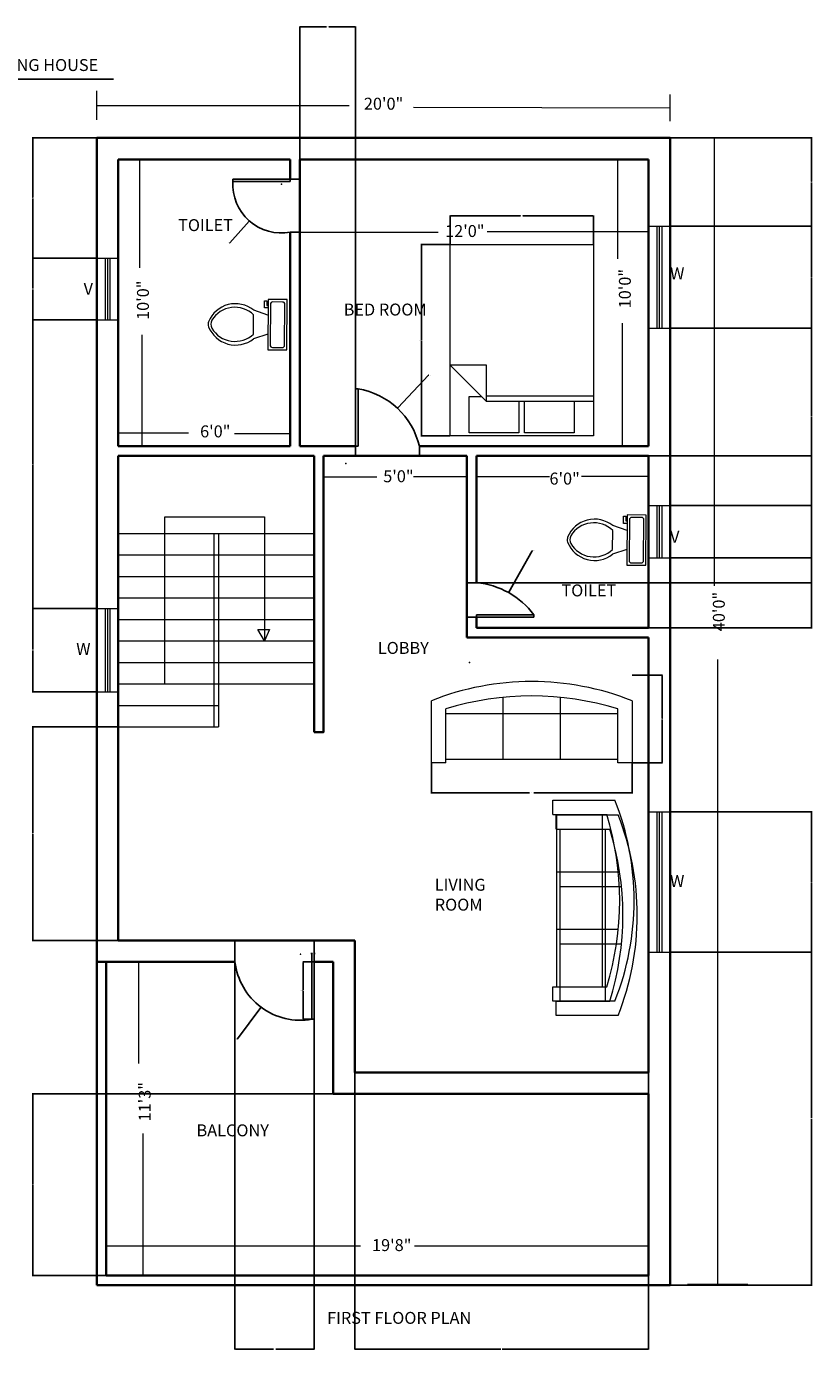
# Model space of a CAD drawing. Units: inches. Extents: x 37 to 686, y -425 to 128.
# Tile 3 of 3: x 357 to 686, y -425 to 128. Entities that reach past the tile are written whole.
import ezdxf

# ---------------------------------------------------------------- set-up
doc = ezdxf.new("R2010")
doc.units = ezdxf.units.IN
doc.header["$MEASUREMENT"] = 0
for name, color, linetype, lineweight in [('A-ANNO-DIMS', 2, 'Continuous', 13), ('A-ANNO-SYMB', 7, 'Continuous', 13), ('A-ANNO-TEXT', 7, 'Continuous', 18), ('A-ANNO-TITL', 7, 'Continuous', 25), ('A-AREA-IDEN', 7, 'Continuous', 18), ('A-DOOR', 3, 'Continuous', 25), ('A-FLOR-FIXT', 9, 'Continuous', 18), ('A-FLOR-STRS', 7, 'Continuous', 20), ('A-FURN', 8, 'Continuous', 18), ('A-GLAZ', 4, 'Continuous', 18), ('A-WALL', 7, 'Continuous', 35)]:
    doc.layers.add(name, color=color, linetype=linetype, lineweight=lineweight)
doc.styles.get("Standard").update_dxf_attribs({"font": 'arial.ttf'})
doc.dimstyles.get("Standard").update_dxf_attribs({"dimtxt": 0.18, "dimasz": 0.18, "dimexe": 0.18, "dimexo": 0.0625, "dimgap": 0.09, "dimtad": 0, "dimtih": 1, "dimtoh": 1, "dimdec": 4, "dimzin": 0, "dimdsep": 46, "dimtxsty": 'Standard', "dimcen": 0.09, "dimadec": 0, "dimazin": 0, "dimtfac": 1, "dimtdec": 4, "dimtofl": 0, "dimtmove": 0, "dimatfit": 3, "dimfxl": 1, "dimtolj": 1, "dimtzin": 0, "dimarcsym": 0})

# ---------------------------------------------------------------- blocks, each defined once
blk = doc.blocks.new('Bed - Queen')
for p, q in [((0, -80.00003), (0, 0)), ((0, 0), (59.99999, 0)), ((59.99999, 0), (59.99999, -80.00003)), ((7.99999, -1.2), (28.79998, -1.2)), ((7.99999, -14.4), (7.99999, -1.2)), ((28.79998, -1.2), (28.79998, -14.4)), ((31.19999, -1.2), (51.99999, -1.2)), ((31.19999, -14.4), (31.19999, -1.2)), ((51.99999, -1.2), (51.99999, -16.4)), ((0, -14.4), (44.8, -14.4)), ((59.99999, -29.6), (44.8, -14.4)), ((44.8, -14.4), (44.8, -29.6)), ((51.99999, -16.4), (46.79936, -16.4)), ((44.8, -16.8), (0, -16.8)), ((44.8, -29.6), (59.99999, -29.6)), ((59.99999, -80.00003), (0, -80.00003))]:
    blk.add_line(p, q)
blk = doc.blocks.new('Sofa - Roundback 7 ft.')
for p, q in [((-12.00002, -32.4421), (-12.00003, -6.5971)), ((11.99997, -32.4421), (11.99998, -6.5971)), ((-36.000027, -34), (-36.000027, -11.4696)), ((-35.999844, -13.3819), (35.9998, -13.3819)), ((35.99998, -34), (35.99998, -11.4696)), ((-36.000027, -32.4421), (35.99998, -32.4421))]:
    blk.add_line(p, q)
for points in [[(-36.000027, -34), (-42.000027, -34), (-42.000027, -8)], [(41.99998, -8), (41.99998, -34), (35.99998, -34)]]:
    blk.add_lwpolyline(points)
for centre, radius, start, end in [((0, -114.25), 114.25, 68.43141, 111.5686), ((-0.00001, -127.1968), 121.1968, 72.72033, 107.2797)]:
    blk.add_arc(centre, radius, start, end)
blk = doc.blocks.new('Toilet - top')
for p, q in [((9.5, -6), (9.5, -2)), ((-10, -8.5), (-8, -8.5)), ((-10, -9.5), (-10, -8.5)), ((-7, -9.5), (-10, -9.5)), ((-8, -8.5), (-8, -8)), ((-7, -8), (-7, -9.5)), ((-4, -8), (-6, -14)), ((4, -8), (6, -14)), ((4, -14), (-4, -14))]:
    blk.add_line(p, q)
blk.add_lwpolyline([(10.5, -8), (10.5, 0), (-10.5, 0), (-10.5, -8)], close=True)
for points in [[(-9.5, -2), (-9.5, -6)], [(8.5, -1), (-8.5, -1)], [(-8.5, -7), (8.5, -7)]]:
    blk.add_lwpolyline(points)
for centre, radius, start, end in [((-8.62, -1.88), 0.884, 81.8699, 188.1301), ((8.62, -1.88), 0.884, 351.8699, 98.1301), ((-8.62, -6.12), 0.884, 171.8699, 278.1301), ((8.62, -6.12), 0.884, 261.8699, 8.1301), ((3.52, -21.58), 12.17, 141.4691, 247.9714), ((4.2, -21.82), 11.33, 136.3677, 238.9468), ((-3.52, -21.58), 12.17, 292.0284, 38.5307), ((-4.2, -21.82), 11.33, 301.053, 43.6321), ((0, -27.88), 4, 245.7318, 294.2682), ((0, -29), 4, 254.8605, 285.1395)]:
    blk.add_arc(centre, radius, start, end)
blk = doc.blocks.new('DOOR-LEAF-24IN')
for p, q in [((0, 0), (0, 24)), ((0, 24), (1, 24)), ((1, 24), (1, 0)), ((1, 0), (0, 0))]:
    blk.add_line(p, q)
blk = doc.blocks.new('*D8')
at = {"layer": 'A-ANNO-DIMS', "color": 0, "lineweight": -2, "transparency": 16777216}
for p, q in [((534.26, 37.12), (522.14, 37.12)), ((522.32, 36.94), (522.32, -2.7)), ((522.32, -42.7), (522.32, -3.06)), ((534.26, -42.88), (522.14, -42.88))]:
    blk.add_line(p, q, dxfattribs=at)
at = {"layer": 'A-ANNO-DIMS', "color": 0, "transparency": 16777216}
for points in [[(522.29, 36.94), (522.35, 36.94), (522.32, 37.12)], [(522.29, -42.7), (522.35, -42.7), (522.32, -42.88)]]:
    blk.add_solid(points, dxfattribs=at)
at = {"layer": 'Defpoints', "color": 0, "transparency": 16777216}
for p in [(534.32, 37.12), (522.32, -42.88), (534.32, -42.88)]:
    blk.add_point(p, dxfattribs=at)
at = {"layer": 'A-ANNO-DIMS', "color": 0, "transparency": 16777216, "insert": (522.32, -2.88), "char_height": 0.18, "attachment_point": 5}
blk.add_mtext('\\A1;BED 80 TYP.', dxfattribs=at)
blk = doc.blocks.new('*D9')
at = {"layer": 'A-ANNO-DIMS', "color": 0, "lineweight": -2, "transparency": 16777216}
for p, q in [((534.32, 37.18), (534.32, 49.3)), ((534.5, 49.12), (563.79, 49.12)), ((594.14, 49.12), (564.85, 49.12)), ((594.32, 37.18), (594.32, 49.3))]:
    blk.add_line(p, q, dxfattribs=at)
at = {"layer": 'A-ANNO-DIMS', "color": 0, "transparency": 16777216}
for points in [[(534.5, 49.15), (534.5, 49.09), (534.32, 49.12)], [(594.14, 49.15), (594.14, 49.09), (594.32, 49.12)]]:
    blk.add_solid(points, dxfattribs=at)
at = {"layer": 'Defpoints', "color": 0, "transparency": 16777216}
for p in [(534.32, 49.12), (534.32, 37.12), (594.32, 37.12)]:
    blk.add_point(p, dxfattribs=at)
at = {"layer": 'A-ANNO-DIMS', "color": 0, "transparency": 16777216, "insert": (564.32, 49.12), "char_height": 0.18, "attachment_point": 5}
blk.add_mtext('\\A1;60 TYP.', dxfattribs=at)
blk = doc.blocks.new('*D12')
at = {"layer": 'A-ANNO-DIMS', "color": 0, "lineweight": -2, "transparency": 16777216}
for p, q in [((476.39, -263), (472.67, -263)), ((472.85, -263.18), (472.85, -274.81)), ((472.85, -286.82), (472.85, -275.18)), ((476.39, -287), (472.67, -287))]:
    blk.add_line(p, q, dxfattribs=at)
at = {"layer": 'A-ANNO-DIMS', "color": 0, "transparency": 16777216}
for points in [[(472.82, -263.18), (472.88, -263.18), (472.85, -263)], [(472.82, -286.82), (472.88, -286.82), (472.85, -287)]]:
    blk.add_solid(points, dxfattribs=at)
at = {"layer": 'Defpoints', "color": 0, "transparency": 16777216}
for p in [(476.45, -263), (472.85, -287), (476.45, -287)]:
    blk.add_point(p, dxfattribs=at)
at = {"layer": 'A-ANNO-DIMS', "color": 0, "transparency": 16777216, "insert": (472.85, -275), "char_height": 0.18, "attachment_point": 5}
blk.add_mtext('\\A1;DOOR LEAF 24 TYP.', dxfattribs=at)
blk = doc.blocks.new('*D13')
at = {"layer": 'A-ANNO-DIMS', "color": 0, "lineweight": -2, "transparency": 16777216}
for p, q in [((476.27, -259.4), (476.09, -259.4)), ((476.45, -262.93), (476.45, -259.22)), ((477.45, -262.93), (477.45, -259.22)), ((477.63, -259.4), (477.81, -259.4))]:
    blk.add_line(p, q, dxfattribs=at)
at = {"layer": 'A-ANNO-DIMS', "color": 0, "transparency": 16777216}
for points in [[(476.27, -259.37), (476.27, -259.43), (476.45, -259.4)], [(477.63, -259.37), (477.63, -259.43), (477.45, -259.4)]]:
    blk.add_solid(points, dxfattribs=at)
at = {"layer": 'Defpoints', "color": 0, "transparency": 16777216}
for p in [(476.45, -259.4), (476.45, -263), (477.45, -263)]:
    blk.add_point(p, dxfattribs=at)
at = {"layer": 'A-ANNO-DIMS', "color": 0, "transparency": 16777216, "insert": (476.95, -259.4), "char_height": 0.18, "attachment_point": 5}
blk.add_mtext('\\A1;1 TYP.', dxfattribs=at)
blk = doc.blocks.new('*D14')
at = {"layer": 'A-ANNO-DIMS', "color": 0, "lineweight": -2, "transparency": 16777216}
for p, q in [((526.49, -179.75), (526.49, -192.47)), ((610.49, -179.75), (610.49, -192.47)), ((526.67, -192.29), (567.59, -192.29)), ((610.31, -192.29), (569.4, -192.29))]:
    blk.add_line(p, q, dxfattribs=at)
at = {"layer": 'A-ANNO-DIMS', "color": 0, "transparency": 16777216}
for points in [[(526.67, -192.26), (526.67, -192.32), (526.49, -192.29)], [(610.31, -192.26), (610.31, -192.32), (610.49, -192.29)]]:
    blk.add_solid(points, dxfattribs=at)
at = {"layer": 'Defpoints', "color": 0, "transparency": 16777216}
for p in [(526.49, -179.69), (610.49, -179.69), (610.49, -192.29)]:
    blk.add_point(p, dxfattribs=at)
at = {"layer": 'A-ANNO-DIMS', "color": 0, "transparency": 16777216, "insert": (568.49, -192.29), "char_height": 0.18, "attachment_point": 5}
blk.add_mtext('\\A1;SOFA 84 TYP.', dxfattribs=at)
blk = doc.blocks.new('*D15')
at = {"layer": 'A-ANNO-DIMS', "color": 0, "lineweight": -2, "transparency": 16777216}
for p, q in [((610.55, -143.02), (623.27, -143.02)), ((623.09, -143.2), (623.09, -161.18)), ((623.09, -179.51), (623.09, -161.54)), ((610.55, -179.69), (623.27, -179.69))]:
    blk.add_line(p, q, dxfattribs=at)
at = {"layer": 'A-ANNO-DIMS', "color": 0, "transparency": 16777216}
for points in [[(623.06, -143.2), (623.12, -143.2), (623.09, -143.02)], [(623.06, -179.51), (623.12, -179.51), (623.09, -179.69)]]:
    blk.add_solid(points, dxfattribs=at)
at = {"layer": 'Defpoints', "color": 0, "transparency": 16777216}
for p in [(610.49, -143.02), (623.09, -143.02), (610.49, -179.69)]:
    blk.add_point(p, dxfattribs=at)
at = {"layer": 'A-ANNO-DIMS', "color": 0, "transparency": 16777216, "insert": (623.09, -161.36), "char_height": 0.18, "attachment_point": 5}
blk.add_mtext('\\A1;37 TYP.', dxfattribs=at)
blk = doc.blocks.new('*D26')
at = {"layer": 'A-ANNO-DIMS', "color": 0, "lineweight": -2, "transparency": 16777216}
for p, q in [((617.35, -318.23), (359.48, -318.23)), ((359.66, -318.41), (359.66, -356.05)), ((359.66, -394.05), (359.66, -356.41)), ((617.35, -394.23), (359.48, -394.23))]:
    blk.add_line(p, q, dxfattribs=at)
at = {"layer": 'A-ANNO-DIMS', "color": 0, "transparency": 16777216}
for points in [[(359.63, -318.41), (359.69, -318.41), (359.66, -318.23)], [(359.63, -394.05), (359.69, -394.05), (359.66, -394.23)]]:
    blk.add_solid(points, dxfattribs=at)
at = {"layer": 'Defpoints', "color": 0, "transparency": 16777216}
for p in [(617.41, -318.23), (359.66, -394.23), (617.41, -394.23)]:
    blk.add_point(p, dxfattribs=at)
at = {"layer": 'A-ANNO-DIMS', "color": 0, "transparency": 16777216, "insert": (359.66, -356.23), "char_height": 0.18, "attachment_point": 5}
blk.add_mtext('\\A1;76', dxfattribs=at)
blk = doc.blocks.new('*D27')
at = {"layer": 'A-ANNO-DIMS', "color": 0, "lineweight": -2, "transparency": 16777216}
for p, q in [((494.42, -309.29), (494.42, -425.16)), ((617.41, -309.29), (617.41, -425.16)), ((494.6, -424.98), (555.64, -424.98)), ((617.23, -424.98), (556.2, -424.98))]:
    blk.add_line(p, q, dxfattribs=at)
at = {"layer": 'A-ANNO-DIMS', "color": 0, "transparency": 16777216}
for points in [[(494.6, -424.95), (494.6, -425.01), (494.42, -424.98)], [(617.23, -424.95), (617.23, -425.01), (617.41, -424.98)]]:
    blk.add_solid(points, dxfattribs=at)
at = {"layer": 'Defpoints', "color": 0, "transparency": 16777216}
for p in [(494.42, -309.23), (617.41, -309.23), (617.41, -424.98)]:
    blk.add_point(p, dxfattribs=at)
at = {"layer": 'A-ANNO-DIMS', "color": 0, "transparency": 16777216, "insert": (555.92, -424.98), "char_height": 0.18, "attachment_point": 5}
blk.add_mtext('\\A1;123', dxfattribs=at)
blk = doc.blocks.new('*D28')
at = {"layer": 'A-ANNO-DIMS', "color": 0, "lineweight": -2, "transparency": 16777216}
for p, q in [((617.47, -51.23), (685.85, -51.23)), ((685.67, -51.41), (685.67, -87.05)), ((685.67, -123.05), (685.67, -87.41)), ((617.47, -123.23), (685.85, -123.23))]:
    blk.add_line(p, q, dxfattribs=at)
at = {"layer": 'A-ANNO-DIMS', "color": 0, "transparency": 16777216}
for points in [[(685.64, -51.41), (685.7, -51.41), (685.67, -51.23)], [(685.64, -123.05), (685.7, -123.05), (685.67, -123.23)]]:
    blk.add_solid(points, dxfattribs=at)
at = {"layer": 'Defpoints', "color": 0, "transparency": 16777216}
for p in [(617.41, -51.23), (617.41, -123.23), (685.67, -123.23)]:
    blk.add_point(p, dxfattribs=at)
at = {"layer": 'A-ANNO-DIMS', "color": 0, "transparency": 16777216, "insert": (685.67, -87.23), "char_height": 0.18, "attachment_point": 5}
blk.add_mtext('\\A1;72', dxfattribs=at)
blk = doc.blocks.new('*D36')
at = {"layer": 'A-ANNO-DIMS', "color": 0, "lineweight": -2, "transparency": 16777216}
for p, q in [((386.35, -115.05), (359.48, -115.05)), ((359.66, -115.23), (359.66, -132.33)), ((359.66, -149.79), (359.66, -132.69)), ((386.35, -149.97), (359.48, -149.97))]:
    blk.add_line(p, q, dxfattribs=at)
at = {"layer": 'A-ANNO-DIMS', "color": 0, "transparency": 16777216}
for points in [[(359.63, -115.23), (359.69, -115.23), (359.66, -115.05)], [(359.63, -149.79), (359.69, -149.79), (359.66, -149.97)]]:
    blk.add_solid(points, dxfattribs=at)
at = {"layer": 'Defpoints', "color": 0, "transparency": 16777216}
for p in [(359.66, -115.05), (386.41, -115.05), (386.41, -149.97)]:
    blk.add_point(p, dxfattribs=at)
at = {"layer": 'A-ANNO-DIMS', "color": 0, "transparency": 16777216, "insert": (359.66, -132.51), "char_height": 0.18, "attachment_point": 5}
blk.add_mtext('\\A1;34.91', dxfattribs=at)
blk = doc.blocks.new('*D37')
at = {"layer": 'A-ANNO-DIMS', "color": 0, "lineweight": -2, "transparency": 16777216}
for p, q in [((386.35, 31.44), (359.48, 31.44)), ((359.66, 31.26), (359.66, 18.71)), ((359.66, 5.8), (359.66, 18.35)), ((386.35, 5.62), (359.48, 5.62))]:
    blk.add_line(p, q, dxfattribs=at)
at = {"layer": 'A-ANNO-DIMS', "color": 0, "transparency": 16777216}
for points in [[(359.63, 31.26), (359.69, 31.26), (359.66, 31.44)], [(359.63, 5.8), (359.69, 5.8), (359.66, 5.62)]]:
    blk.add_solid(points, dxfattribs=at)
at = {"layer": 'Defpoints', "color": 0, "transparency": 16777216}
for p in [(359.66, 31.44), (386.41, 31.44), (386.41, 5.62)]:
    blk.add_point(p, dxfattribs=at)
at = {"layer": 'A-ANNO-DIMS', "color": 0, "transparency": 16777216, "insert": (359.66, 18.53), "char_height": 0.18, "attachment_point": 5}
blk.add_mtext('\\A1;25.823', dxfattribs=at)
blk = doc.blocks.new('*D38')
at = {"layer": 'A-ANNO-DIMS', "color": 0, "lineweight": -2, "transparency": 16777216}
for p, q in [((626.47, 44.9), (685.85, 44.9)), ((685.67, 44.72), (685.67, 23.7)), ((685.67, 2.31), (685.67, 23.34)), ((626.47, 2.13), (685.85, 2.13))]:
    blk.add_line(p, q, dxfattribs=at)
at = {"layer": 'A-ANNO-DIMS', "color": 0, "transparency": 16777216}
for points in [[(685.64, 44.72), (685.7, 44.72), (685.67, 44.9)], [(685.64, 2.31), (685.7, 2.31), (685.67, 2.13)]]:
    blk.add_solid(points, dxfattribs=at)
at = {"layer": 'Defpoints', "color": 0, "transparency": 16777216}
for p in [(626.41, 44.9), (685.67, 44.9), (626.41, 2.13)]:
    blk.add_point(p, dxfattribs=at)
at = {"layer": 'A-ANNO-DIMS', "color": 0, "transparency": 16777216, "insert": (685.67, 23.52), "char_height": 0.18, "attachment_point": 5}
blk.add_mtext('\\A1;42.77', dxfattribs=at)
blk = doc.blocks.new('*D39')
at = {"layer": 'A-ANNO-DIMS', "color": 0, "lineweight": -2, "transparency": 16777216}
for p, q in [((626.47, -71.98), (685.85, -71.98)), ((685.67, -72.16), (685.67, -82.77)), ((685.67, -93.75), (685.67, -83.14)), ((626.47, -93.93), (685.85, -93.93))]:
    blk.add_line(p, q, dxfattribs=at)
at = {"layer": 'A-ANNO-DIMS', "color": 0, "transparency": 16777216}
for points in [[(685.64, -72.16), (685.7, -72.16), (685.67, -71.98)], [(685.64, -93.75), (685.7, -93.75), (685.67, -93.93)]]:
    blk.add_solid(points, dxfattribs=at)
at = {"layer": 'Defpoints', "color": 0, "transparency": 16777216}
for p in [(626.41, -71.98), (626.41, -93.93), (685.67, -93.93)]:
    blk.add_point(p, dxfattribs=at)
at = {"layer": 'A-ANNO-DIMS', "color": 0, "transparency": 16777216, "insert": (685.67, -82.95), "char_height": 0.18, "attachment_point": 5}
blk.add_mtext('\\A1;21.946', dxfattribs=at)
blk = doc.blocks.new('*D40')
at = {"layer": 'A-ANNO-DIMS', "color": 0, "lineweight": -2, "transparency": 16777216}
for p, q in [((626.47, -200.25), (685.85, -200.25)), ((685.67, -200.43), (685.67, -229.42)), ((685.67, -258.77), (685.67, -229.79)), ((626.47, -258.95), (685.85, -258.95))]:
    blk.add_line(p, q, dxfattribs=at)
at = {"layer": 'A-ANNO-DIMS', "color": 0, "transparency": 16777216}
for points in [[(685.64, -200.43), (685.7, -200.43), (685.67, -200.25)], [(685.64, -258.77), (685.7, -258.77), (685.67, -258.95)]]:
    blk.add_solid(points, dxfattribs=at)
at = {"layer": 'Defpoints', "color": 0, "transparency": 16777216}
for p in [(626.41, -200.25), (685.67, -200.25), (626.41, -258.95)]:
    blk.add_point(p, dxfattribs=at)
at = {"layer": 'A-ANNO-DIMS', "color": 0, "transparency": 16777216, "insert": (685.67, -229.6), "char_height": 0.18, "attachment_point": 5}
blk.add_mtext('\\A1;58.7', dxfattribs=at)
blk = doc.blocks.new('*D48')
at = {"layer": 'A-ANNO-DIMS', "color": 0, "lineweight": -2, "transparency": 16777216}
for p, q in [((386.35, 81.77), (359.48, 81.77)), ((359.66, 81.59), (359.66, 56.79)), ((359.66, 31.62), (359.66, 56.42)), ((386.35, 31.44), (359.48, 31.44))]:
    blk.add_line(p, q, dxfattribs=at)
at = {"layer": 'A-ANNO-DIMS', "color": 0, "transparency": 16777216}
for points in [[(359.63, 81.59), (359.69, 81.59), (359.66, 81.77)], [(359.63, 31.62), (359.69, 31.62), (359.66, 31.44)]]:
    blk.add_solid(points, dxfattribs=at)
at = {"layer": 'Defpoints', "color": 0, "transparency": 16777216}
for p in [(359.66, 81.77), (386.41, 81.77), (386.41, 31.44)]:
    blk.add_point(p, dxfattribs=at)
at = {"layer": 'A-ANNO-DIMS', "color": 0, "transparency": 16777216, "insert": (359.66, 56.61), "char_height": 0.18, "attachment_point": 5}
blk.add_mtext('\\A1;50.33', dxfattribs=at)
blk = doc.blocks.new('*D49')
at = {"layer": 'A-ANNO-DIMS', "color": 0, "lineweight": -2, "transparency": 16777216}
for p, q in [((386.35, 5.62), (359.48, 5.62)), ((359.66, 5.44), (359.66, -54.54)), ((359.66, -114.87), (359.66, -54.9)), ((386.35, -115.05), (359.48, -115.05))]:
    blk.add_line(p, q, dxfattribs=at)
at = {"layer": 'A-ANNO-DIMS', "color": 0, "transparency": 16777216}
for points in [[(359.63, 5.44), (359.69, 5.44), (359.66, 5.62)], [(359.63, -114.87), (359.69, -114.87), (359.66, -115.05)]]:
    blk.add_solid(points, dxfattribs=at)
at = {"layer": 'Defpoints', "color": 0, "transparency": 16777216}
for p in [(359.66, 5.62), (386.41, 5.62), (386.41, -115.05)]:
    blk.add_point(p, dxfattribs=at)
at = {"layer": 'A-ANNO-DIMS', "color": 0, "transparency": 16777216, "insert": (359.66, -54.72), "char_height": 0.18, "attachment_point": 5}
blk.add_mtext('\\A1;120.67', dxfattribs=at)
blk = doc.blocks.new('*D50')
at = {"layer": 'A-ANNO-DIMS', "color": 0, "lineweight": -2, "transparency": 16777216}
for p, q in [((626.47, 81.77), (685.85, 81.77)), ((685.67, 81.59), (685.67, 63.52)), ((685.67, 45.08), (685.67, 63.16)), ((626.47, 44.9), (685.85, 44.9))]:
    blk.add_line(p, q, dxfattribs=at)
at = {"layer": 'A-ANNO-DIMS', "color": 0, "transparency": 16777216}
for points in [[(685.64, 81.59), (685.7, 81.59), (685.67, 81.77)], [(685.64, 45.08), (685.7, 45.08), (685.67, 44.9)]]:
    blk.add_solid(points, dxfattribs=at)
at = {"layer": 'Defpoints', "color": 0, "transparency": 16777216}
for p in [(626.41, 81.77), (685.67, 81.77), (626.41, 44.9)]:
    blk.add_point(p, dxfattribs=at)
at = {"layer": 'A-ANNO-DIMS', "color": 0, "transparency": 16777216, "insert": (685.67, 63.34), "char_height": 0.18, "attachment_point": 5}
blk.add_mtext('\\A1;36.87', dxfattribs=at)
blk = doc.blocks.new('*D51')
at = {"layer": 'A-ANNO-DIMS', "color": 0, "lineweight": -2, "transparency": 16777216}
for p, q in [((626.47, 2.13), (685.85, 2.13)), ((685.67, 1.95), (685.67, -34.74)), ((685.67, -71.8), (685.67, -35.1)), ((626.47, -71.98), (685.85, -71.98))]:
    blk.add_line(p, q, dxfattribs=at)
at = {"layer": 'A-ANNO-DIMS', "color": 0, "transparency": 16777216}
for points in [[(685.64, 1.95), (685.7, 1.95), (685.67, 2.13)], [(685.64, -71.8), (685.7, -71.8), (685.67, -71.98)]]:
    blk.add_solid(points, dxfattribs=at)
at = {"layer": 'Defpoints', "color": 0, "transparency": 16777216}
for p in [(626.41, 2.13), (685.67, 2.13), (626.41, -71.98)]:
    blk.add_point(p, dxfattribs=at)
at = {"layer": 'A-ANNO-DIMS', "color": 0, "transparency": 16777216, "insert": (685.67, -34.92), "char_height": 0.18, "attachment_point": 5}
blk.add_mtext('\\A1;74.11', dxfattribs=at)
blk = doc.blocks.new('*D52')
at = {"layer": 'A-ANNO-DIMS', "color": 0, "lineweight": -2, "transparency": 16777216}
for p, q in [((626.47, -258.95), (685.85, -258.95)), ((685.67, -259.13), (685.67, -328.41)), ((685.67, -398.05), (685.67, -328.77)), ((626.47, -398.23), (685.85, -398.23))]:
    blk.add_line(p, q, dxfattribs=at)
at = {"layer": 'A-ANNO-DIMS', "color": 0, "transparency": 16777216}
for points in [[(685.64, -259.13), (685.7, -259.13), (685.67, -258.95)], [(685.64, -398.05), (685.7, -398.05), (685.67, -398.23)]]:
    blk.add_solid(points, dxfattribs=at)
at = {"layer": 'Defpoints', "color": 0, "transparency": 16777216}
for p in [(626.41, -258.95), (685.67, -258.95), (626.41, -398.23)]:
    blk.add_point(p, dxfattribs=at)
at = {"layer": 'A-ANNO-DIMS', "color": 0, "transparency": 16777216, "insert": (685.67, -328.59), "char_height": 0.18, "attachment_point": 5}
blk.add_mtext('\\A1;139.27', dxfattribs=at)
blk = doc.blocks.new('*D55')
at = {"layer": 'A-ANNO-DIMS', "color": 0, "lineweight": -2, "transparency": 16777216}
for p, q in [((444.29, -263.06), (444.29, -425.16)), ((477.45, -263.06), (477.45, -425.16)), ((444.47, -424.98), (460.41, -424.98)), ((477.27, -424.98), (461.34, -424.98))]:
    blk.add_line(p, q, dxfattribs=at)
at = {"layer": 'A-ANNO-DIMS', "color": 0, "transparency": 16777216}
for points in [[(444.47, -424.95), (444.47, -425.01), (444.29, -424.98)], [(477.27, -424.95), (477.27, -425.01), (477.45, -424.98)]]:
    blk.add_solid(points, dxfattribs=at)
at = {"layer": 'Defpoints', "color": 0, "transparency": 16777216}
for p in [(444.29, -263), (477.45, -263), (477.45, -424.98)]:
    blk.add_point(p, dxfattribs=at)
at = {"layer": 'A-ANNO-DIMS', "color": 0, "transparency": 16777216, "insert": (460.87, -424.98), "char_height": 0.18, "attachment_point": 5}
blk.add_mtext('\\A1;33.156', dxfattribs=at)
blk = doc.blocks.new('*D56')
at = {"layer": 'A-ANNO-DIMS', "color": 0, "lineweight": -2, "transparency": 16777216}
for p, q in [((395.35, -164.68), (359.48, -164.68)), ((359.66, -164.86), (359.66, -209.15)), ((359.66, -253.82), (359.66, -209.52)), ((395.35, -254), (359.48, -254))]:
    blk.add_line(p, q, dxfattribs=at)
at = {"layer": 'A-ANNO-DIMS', "color": 0, "transparency": 16777216}
for points in [[(359.63, -164.86), (359.69, -164.86), (359.66, -164.68)], [(359.63, -253.82), (359.69, -253.82), (359.66, -254)]]:
    blk.add_solid(points, dxfattribs=at)
at = {"layer": 'Defpoints', "color": 0, "transparency": 16777216}
for p in [(359.66, -164.68), (395.41, -164.68), (395.41, -254)]:
    blk.add_point(p, dxfattribs=at)
at = {"layer": 'A-ANNO-DIMS', "color": 0, "transparency": 16777216, "insert": (359.66, -209.34), "char_height": 0.18, "attachment_point": 5}
blk.add_mtext('\\A1;89.32', dxfattribs=at)
blk = doc.blocks.new('*D60')
at = {"layer": 'A-ANNO-DIMS', "color": 0, "lineweight": -2, "transparency": 16777216}
for p, q in [((471.41, -47.16), (471.41, 128.4)), ((471.59, 128.22), (482.64, 128.22)), ((494.62, 128.22), (483.57, 128.22)), ((494.8, -47.16), (494.8, 128.4))]:
    blk.add_line(p, q, dxfattribs=at)
at = {"layer": 'A-ANNO-DIMS', "color": 0, "transparency": 16777216}
for points in [[(471.59, 128.25), (471.59, 128.19), (471.41, 128.22)], [(494.62, 128.25), (494.62, 128.19), (494.8, 128.22)]]:
    blk.add_solid(points, dxfattribs=at)
at = {"layer": 'Defpoints', "color": 0, "transparency": 16777216}
for p in [(494.8, 128.22), (471.41, -47.23), (494.8, -47.23)]:
    blk.add_point(p, dxfattribs=at)
at = {"layer": 'A-ANNO-DIMS', "color": 0, "transparency": 16777216, "insert": (483.1, 128.22), "char_height": 0.18, "attachment_point": 5}
blk.add_mtext('\\A1;23.386', dxfattribs=at)
blk = doc.blocks.new('*D61')
at = {"layer": 'A-ANNO-DIMS', "color": 0, "lineweight": -2, "transparency": 16777216}
for p, q in [((545.47, -51.23), (685.85, -51.23)), ((685.67, -51.41), (685.67, -77.59)), ((685.67, -104.14), (685.67, -77.95)), ((545.47, -104.32), (685.85, -104.32))]:
    blk.add_line(p, q, dxfattribs=at)
at = {"layer": 'A-ANNO-DIMS', "color": 0, "transparency": 16777216}
for points in [[(685.64, -51.41), (685.7, -51.41), (685.67, -51.23)], [(685.64, -104.14), (685.7, -104.14), (685.67, -104.32)]]:
    blk.add_solid(points, dxfattribs=at)
at = {"layer": 'Defpoints', "color": 0, "transparency": 16777216}
for p in [(545.41, -51.23), (545.41, -104.32), (685.67, -104.32)]:
    blk.add_point(p, dxfattribs=at)
at = {"layer": 'A-ANNO-DIMS', "color": 0, "transparency": 16777216, "insert": (685.67, -77.77), "char_height": 0.18, "attachment_point": 5}
blk.add_mtext('\\A1;53.09', dxfattribs=at)
blk = doc.blocks.new('*D63')
at = {"layer": 'A-ANNO-DIMS', "color": 0, "lineweight": -2, "transparency": 16777216}
for p, q in [((568.71, -90.95), (558.95, -108.33)), ((568.89, -90.95), (568.71, -90.95)), ((542.35, -137.71), (542.53, -137.71)), ((542.44, -137.8), (542.44, -137.62))]:
    blk.add_line(p, q, dxfattribs=at)
at = {"layer": 'A-ANNO-DIMS', "color": 0, "transparency": 16777216}
blk.add_solid([(558.92, -108.31), (558.97, -108.34), (558.86, -108.48)], dxfattribs=at)
at = {"layer": 'Defpoints', "color": 0, "transparency": 16777216}
for p in [(558.86, -108.48), (542.44, -137.71)]:
    blk.add_point(p, dxfattribs=at)
at = {"layer": 'A-ANNO-DIMS', "color": 0, "transparency": 16777216, "insert": (569.37, -90.95), "char_height": 0.18, "attachment_point": 5}
blk.add_mtext('\\A1;R33.52', dxfattribs=at)
blk = doc.blocks.new('*D65')
at = {"layer": 'A-ANNO-DIMS', "color": 0, "lineweight": -2, "transparency": 16777216}
for p, q in [((525.24, -17.46), (512.41, -31.2)), ((525.42, -17.46), (525.24, -17.46)), ((490.61, -54.44), (490.79, -54.44)), ((490.7, -54.53), (490.7, -54.35))]:
    blk.add_line(p, q, dxfattribs=at)
at = {"layer": 'A-ANNO-DIMS', "color": 0, "transparency": 16777216}
blk.add_solid([(512.39, -31.18), (512.43, -31.22), (512.29, -31.33)], dxfattribs=at)
at = {"layer": 'Defpoints', "color": 0, "transparency": 16777216}
for p in [(512.29, -31.33), (490.7, -54.44)]:
    blk.add_point(p, dxfattribs=at)
at = {"layer": 'A-ANNO-DIMS', "color": 0, "transparency": 16777216, "insert": (525.9, -17.46), "char_height": 0.18, "attachment_point": 5}
blk.add_mtext('\\A1;R31.62', dxfattribs=at)
blk = doc.blocks.new('*D67')
at = {"layer": 'A-ANNO-DIMS', "color": 0, "lineweight": -2, "transparency": 16777216}
for p, q in [((471.65, -259.77), (471.83, -259.77)), ((471.74, -259.86), (471.74, -259.68)), ((445.29, -295.2), (455.1, -282.06)), ((445.11, -295.2), (445.29, -295.2))]:
    blk.add_line(p, q, dxfattribs=at)
at = {"layer": 'A-ANNO-DIMS', "color": 0, "transparency": 16777216}
blk.add_solid([(455.08, -282.04), (455.13, -282.07), (455.21, -281.91)], dxfattribs=at)
at = {"layer": 'Defpoints', "color": 0, "transparency": 16777216}
for p in [(471.74, -259.77), (455.21, -281.91)]:
    blk.add_point(p, dxfattribs=at)
at = {"layer": 'A-ANNO-DIMS', "color": 0, "transparency": 16777216, "insert": (444.63, -295.2), "char_height": 0.18, "attachment_point": 5}
blk.add_mtext('\\A1;R27.63', dxfattribs=at)
blk = doc.blocks.new('*D69')
at = {"layer": 'A-ANNO-DIMS', "color": 0, "lineweight": -2, "transparency": 16777216}
for p, q in [((463.69, 62.4), (463.87, 62.4)), ((463.78, 62.31), (463.78, 62.49)), ((442.19, 37.92), (450.17, 46.96)), ((442.01, 37.92), (442.19, 37.92))]:
    blk.add_line(p, q, dxfattribs=at)
at = {"layer": 'A-ANNO-DIMS', "color": 0, "transparency": 16777216}
blk.add_solid([(450.14, 46.98), (450.19, 46.94), (450.29, 47.1)], dxfattribs=at)
at = {"layer": 'Defpoints', "color": 0, "transparency": 16777216}
for p in [(463.78, 62.4), (450.29, 47.1)]:
    blk.add_point(p, dxfattribs=at)
at = {"layer": 'A-ANNO-DIMS', "color": 0, "transparency": 16777216, "insert": (441.46, 37.92), "char_height": 0.18, "attachment_point": 5}
blk.add_mtext('\\A1;R20.402', dxfattribs=at)

msp = doc.modelspace()

# ---------------------------------------------------------------- linework, layer by layer
at = {"layer": 'A-ANNO-DIMS'}
for p, q in [((386.4114, 89.3296), (386.4114, 101.4672)), ((626.4114, 88.7375), (626.4114, 99.987)), ((386.4114, 95.3984), (492.0307, 95.3984)), ((519.0018, 94.6583), (626.4114, 94.3623)), ((631.909, 81.9543), (657.8745, 81.9543)), ((644.8918, 81.9543), (644.8918, -105.6438)), ((404.4762, 27.441), (404.4762, 72.7729)), ((604.4594, 72.7729), (604.4594, 31.1608)), ((471.4114, 42.3205), (529.3772, 42.3205)), ((549.8488, 42.6387), (617.4114, 42.6387)), ((606.29, 4.1919), (606.29, -47.2271)), ((405.3539, -0.6131), (405.3539, -47.2271)), ((424.7969, -41.7157), (395.4114, -41.7157)), ((444.0844, -41.841), (467.4114, -41.841)), ((481.4114, -60.0408), (503.6246, -60.0408)), ((519.0833, -59.8976), (541.4114, -59.8976)), ((545.4114, -59.8976), (575.9323, -59.8976)), ((589.3506, -59.6849), (617.4114, -59.6849)), ((646.3442, -397.7918), (646.3442, -136.4803)), ((404.018, -305.5393), (404.018, -262.9952)), ((405.7754, -334.764), (405.7754, -381.9605)), ((519.3979, -381.7828), (617.4114, -381.7828)), ((395.4114, -381.9605), (390.4114, -381.9605)), ((496.8886, -381.9605), (395.4114, -381.9605)), ((405.7754, -381.9605), (405.7754, -389.2271)), ((405.7754, -389.2271), (405.7754, -394.2271)), ((633.7697, -397.7918), (658.9186, -397.7918))]:
    msp.add_line(p, q, dxfattribs=at)
at = {"layer": 'A-ANNO-SYMB'}
for p, q in [((414.9345, -146.6754), (414.9345, -76.746)), ((414.9345, -76.746), (456.6656, -76.746)), ((456.6656, -76.746), (456.6656, -128.6754)), ((456.6656, -128.6754), (453.9181, -123.9166)), ((453.9181, -123.9166), (458.8028, -123.9166)), ((458.8028, -123.9166), (456.6656, -128.6754))]:
    msp.add_line(p, q, dxfattribs=at)
at = {"layer": 'A-ANNO-TITL'}
msp.add_line((320.568, 106.3633), (393.4497, 106.3633), dxfattribs=at)
at = {"layer": 'A-DOOR'}
for p, q in [((467.4114, 64.4949), (471.4114, 64.4949)), ((467.4114, 42.3205), (471.4114, 42.3205)), ((494.7972, -51.2271), (494.7972, -47.2271)), ((521.4891, -51.2271), (521.4891, -47.2271)), ((541.4114, -104.3183), (545.4114, -104.3183)), ((541.4114, -118.8056), (545.4114, -118.8056)), ((444.2945, -262.9952), (444.2945, -253.9952)), ((477.4503, -262.9952), (477.4503, -253.9952))]:
    msp.add_line(p, q, dxfattribs=at)
for centre, radius, start, end in [((463.7844, 62.398), 20.4025, 176.918049, 280.240214), ((490.6991, -54.4361), 31.6227, 13.17759, 80.722384), ((542.4368, -137.7087), 33.5226, 36.421615, 84.909158), ((471.7376, -259.7679), 27.6322, 186.707299, 279.819796)]:
    msp.add_arc(centre, radius, start, end, dxfattribs=at)
at = {"layer": 'A-FLOR-STRS'}
for p, q in [((395.4114, -83.6754), (477.4114, -83.6754)), ((435.4114, -83.6754), (435.4114, -164.6754)), ((437.4114, -83.6754), (437.4114, -164.6754)), ((395.4114, -92.6754), (477.4114, -92.6754)), ((395.4114, -101.6754), (477.4114, -101.6754)), ((395.4114, -110.6754), (477.4114, -110.6754)), ((395.4114, -119.6754), (477.4114, -119.6754)), ((395.4114, -128.6754), (477.4114, -128.6754)), ((395.4114, -137.6754), (477.4114, -137.6754)), ((395.4114, -146.6754), (477.4114, -146.6754)), ((395.4114, -155.6754), (437.4114, -155.6754)), ((395.4114, -164.6754), (437.4114, -164.6754))]:
    msp.add_line(p, q, dxfattribs=at)
at = {"layer": 'A-GLAZ'}
for p, q in [((617.4114, 44.9049), (626.4114, 44.9049)), ((620.9114, 44.9049), (620.9114, 2.1316)), ((621.9114, 44.9049), (621.9114, 2.1316)), ((622.9114, 44.9049), (622.9114, 2.1316)), ((386.4114, 31.44), (395.4114, 31.44)), ((389.9114, 31.44), (389.9114, 5.6174)), ((390.9114, 31.44), (390.9114, 5.6174)), ((391.9114, 31.44), (391.9114, 5.6174)), ((386.4114, 5.6174), (395.4114, 5.6174)), ((617.4114, 2.1316), (626.4114, 2.1316)), ((617.4114, -71.9808), (626.4114, -71.9808)), ((620.9114, -71.9808), (620.9114, -93.9265)), ((621.9114, -71.9808), (621.9114, -93.9265)), ((622.9114, -71.9808), (622.9114, -93.9265)), ((617.4114, -93.9265), (626.4114, -93.9265)), ((386.4114, -115.0549), (395.4114, -115.0549)), ((389.9114, -115.0549), (389.9114, -149.9657)), ((390.9114, -115.0549), (390.9114, -149.9657)), ((391.9114, -115.0549), (391.9114, -149.9657)), ((386.4114, -149.9657), (395.4114, -149.9657)), ((617.4114, -200.252), (626.4114, -200.252)), ((620.9114, -200.252), (620.9114, -258.9544)), ((621.9114, -200.252), (621.9114, -258.9544)), ((622.9114, -200.252), (622.9114, -258.9544)), ((617.4114, -258.9544), (626.4114, -258.9544))]:
    msp.add_line(p, q, dxfattribs=at)
at = {"layer": 'A-WALL'}
for p, q in [((386.4114, 81.7729), (626.4114, 81.7729)), ((386.4114, -398.2271), (386.4114, 81.7729)), ((626.4114, 81.7729), (626.4114, -398.2271)), ((395.4114, 72.7729), (467.4114, 72.7729)), ((395.4114, -47.2271), (395.4114, 72.7729)), ((467.4114, 64.4949), (467.4114, 72.7729)), ((471.4114, -47.2271), (471.4114, 72.7729)), ((471.4114, 72.7729), (617.4114, 72.7729)), ((617.4114, 72.7729), (617.4114, -47.2271)), ((467.4114, -47.2271), (467.4114, 42.3205)), ((395.4114, -47.2271), (467.4114, -47.2271)), ((471.4114, -47.2271), (494.7972, -47.2271)), ((521.4891, -47.2271), (617.4114, -47.2271)), ((395.4114, -51.2271), (477.4114, -51.2271)), ((395.4114, -253.9952), (395.4114, -51.2271)), ((477.4114, -51.2271), (477.4114, -127.2271)), ((481.4114, -51.2271), (481.4114, -127.2271)), ((481.4114, -51.2271), (541.4114, -51.2271)), ((541.4114, -51.2271), (541.4114, -127.2271)), ((545.4114, -51.2271), (545.4114, -104.3183)), ((545.4114, -51.2271), (617.4114, -51.2271)), ((617.4114, -51.2271), (617.4114, -123.2271)), ((545.4114, -118.8056), (545.4114, -123.2271)), ((477.4114, -127.2271), (477.4114, -166.8153)), ((541.4114, -127.2271), (617.4114, -127.2271)), ((545.4114, -123.2271), (617.4114, -123.2271)), ((617.4114, -127.2271), (617.4114, -309.2271)), ((395.4114, -253.9952), (494.423, -253.9952)), ((494.423, -253.9952), (494.423, -309.2271)), ((395.4114, -262.9952), (386.4114, -262.9952)), ((390.4114, -394.2271), (390.4114, -262.9952)), ((395.4114, -262.9952), (444.2945, -262.9952)), ((477.4503, -262.9952), (485.423, -262.9952)), ((485.423, -262.9952), (485.423, -309.2271)), ((485.423, -309.2271), (485.423, -318.2271)), ((617.4114, -309.2271), (494.423, -309.2271)), ((617.4114, -318.2271), (485.423, -318.2271)), ((617.4114, -318.2271), (617.4114, -389.2271)), ((617.4114, -389.2271), (617.4114, -394.2271)), ((626.4114, -398.2271), (386.4114, -398.2271)), ((617.4114, -394.2271), (390.4114, -394.2271))]:
    msp.add_line(p, q, dxfattribs=at)
msp.add_lwpolyline([(481.4114, -127.2271), (481.4114, -166.8153), (477.4114, -166.8153)], dxfattribs=at)

# ---------------------------------------------------------------- block references
at = {"layer": 'A-DOOR'}
for p, rotation in [((443.4116, 64.4948), 269.9999999999999), ((569.4113, -118.8054), 89.99999999999984), ((477.4501, -262.9953), 180)]:
    msp.add_blockref('DOOR-LEAF-24IN', p, dxfattribs=dict(at, rotation=rotation))
msp.add_blockref('DOOR-LEAF-24IN', (494.7974, -47.227), dxfattribs=at)
at = {"layer": 'A-FLOR-FIXT', "rotation": 269.5733184257299}
for p in [(466.0881, 3.5942), (616.3761, -86.558)]:
    msp.add_blockref('Toilet - top', p, dxfattribs=at)
at = {"layer": 'A-FURN'}
for name, p, rotation in [('Bed - Queen', (594.3209, -42.8782), 180), ('Sofa - Roundback 7 ft.', (611.3478, -237.3424), 270), ('Sofa - Roundback 7 ft.', (612.6781, -243.4369), 270)]:
    msp.add_blockref(name, p, dxfattribs=dict(at, rotation=rotation))
msp.add_blockref('Sofa - Roundback 7 ft.', (568.4909, -145.6904), dxfattribs=at)

# ---------------------------------------------------------------- texts
at = {"layer": 'A-ANNO-DIMS', "char_height": 5, "attachment_point": 1}
for s, width, insert in [('20\'0"', 66.49393, (498.2548, 98.5799)), ('12\'0"', 35.858568, (532.2586, 45.3112)), ('6\'0"', 27.670391, (429.7013, -38.5194)), ('5\'0"', 20.747672, (506.3583, -57.2907)), ('6\'0"', 27.670391, (575.9323, -58.2717)), ('19\'8"', 40.826541, (501.665, -378.967))]:
    msp.add_mtext_dynamic_manual_height_columns(s, width=width, gutter_width=25, heights=[0], dxfattribs=dict(at, insert=insert))
at = {"layer": 'A-ANNO-DIMS', "char_height": 5, "attachment_point": 1, "rotation": 90}
for s, width, insert in [('10\'0"', 27.842625, (604.9853, 10.4667)), ('10\'0"', 27.842625, (403.2861, 5.6174)), ('40\'0"', 31.535776, (644.3193, -124.6216)), ('11\'3"', 24.184865, (404.018, -329.7241))]:
    msp.add_mtext_dynamic_manual_height_columns(s, width=width, gutter_width=25, heights=[0], dxfattribs=dict(at, insert=insert))
at = {"layer": 'A-ANNO-TEXT', "char_height": 5, "attachment_point": 1}
for s, width, insert in [('W', 8.568355, (626.4114, 27.5575)), ('V', 13.447234, (380.9472, 21.1263)), ('V', 13.447234, (626.4114, -82.6031)), ('W', 8.568355, (377.8535, -129.525)), ('W', 8.568355, (626.4114, -226.6384))]:
    msp.add_mtext_dynamic_manual_height_columns(s, width=width, gutter_width=25, heights=[0], dxfattribs=dict(at, insert=insert))
at = {"layer": 'A-ANNO-TITL', "char_height": 5, "attachment_point": 1}
for s, width, insert in [('EAST FACING HOUSE', 258.611498, (320.7609, 114.7635)), ('FIRST FLOOR PLAN', 184.056372, (482.8707, -409.4107))]:
    msp.add_mtext_dynamic_manual_height_columns(s, width=width, gutter_width=25, heights=[0], dxfattribs=dict(at, insert=insert))
at = {"layer": 'A-AREA-IDEN', "char_height": 5, "attachment_point": 1}
for s, width, insert in [('TOILET', 38.596876, (420.5149, 47.7824)), ('BED ROOM', 83.955241, (489.805, 12.4565)), ('TOILET', 38.596876, (580.9403, -105.0553)), ('LOBBY', 26.091096, (504.0968, -129.1153)), ('LIVING\\PROOM', 48.553453, (527.925, -228.1916)), ('BALCONY', 94.333055, (428.2028, -330.9559))]:
    msp.add_mtext_dynamic_manual_height_columns(s, width=width, gutter_width=25, heights=[0], dxfattribs=dict(at, insert=insert))

# ---------------------------------------------------------------- dimensions: what is measured, and where the dimension line sits
at = {"layer": 'A-ANNO-DIMS'}
for base, p1, p2, override, picture, middle in [((494.7972, 128.2172), (471.4114, -47.2271), (494.7972, -47.2271), {"dimdec": 3, "dimlfac": 1, "dimrnd": 0, "dimzin": 0, "dimdsep": 46, "dimlunit": 2}, '*D60', (483.1043, 128.2172)), ((477.4503, -424.9771), (444.2945, -262.9952), (477.4503, -262.9952), {"dimdec": 3, "dimlfac": 1, "dimrnd": 0, "dimzin": 0, "dimdsep": 46, "dimlunit": 2}, '*D55', (460.8724, -424.9771)), ((617.4114, -424.9771), (494.423, -309.2271), (617.4114, -309.2271), {"dimdec": 0, "dimlfac": 1, "dimrnd": 0, "dimzin": 0, "dimdsep": 46, "dimlunit": 2}, '*D27', (555.9172, -424.9771))]:
    dim = msp.add_linear_dim(base=base, p1=p1, p2=p2, dimstyle='Standard', override=override, dxfattribs=at)
    dim.commit()
    dim.dimension.update_dxf_attribs({"geometry": picture, "text_midpoint": middle})
for base, p1, p2, override, picture, middle in [((359.6614, 81.7729), (386.4114, 31.44), (386.4114, 81.7729), {"dimdec": 2, "dimlfac": 1, "dimrnd": 0, "dimzin": 0, "dimdsep": 46, "dimlunit": 2}, '*D48', (359.6614, 56.6064)), ((685.6686, 81.7729), (626.4114, 44.9049), (626.4114, 81.7729), {"dimdec": 2, "dimlfac": 1, "dimrnd": 0, "dimzin": 0, "dimdsep": 46, "dimlunit": 2}, '*D50', (685.6686, 63.3389)), ((685.6686, 44.9049), (626.4114, 2.1316), (626.4114, 44.9049), {"dimdec": 2, "dimlfac": 1, "dimrnd": 0, "dimzin": 0, "dimdsep": 46, "dimlunit": 2}, '*D38', (685.6686, 23.5183)), ((359.6614, 31.44), (386.4114, 5.6174), (386.4114, 31.44), {"dimdec": 3, "dimlfac": 1, "dimrnd": 0, "dimzin": 0, "dimdsep": 46, "dimlunit": 2}, '*D37', (359.6614, 18.5287)), ((359.6614, 5.6174), (386.4114, -115.0549), (386.4114, 5.6174), {"dimdec": 2, "dimlfac": 1, "dimrnd": 0, "dimzin": 0, "dimdsep": 46, "dimlunit": 2}, '*D49', (359.6614, -54.7187)), ((685.6686, 2.1316), (626.4114, -71.9808), (626.4114, 2.1316), {"dimdec": 2, "dimlfac": 1, "dimrnd": 0, "dimzin": 0, "dimdsep": 46, "dimlunit": 2}, '*D51', (685.6686, -34.9246)), ((685.6686, -104.3183), (545.4114, -51.2271), (545.4114, -104.3183), {"dimdec": 2, "dimlfac": 1, "dimrnd": 0, "dimzin": 0, "dimdsep": 46, "dimlunit": 2}, '*D61', (685.6686, -77.7727)), ((685.6686, -123.2271), (617.4114, -51.2271), (617.4114, -123.2271), {"dimdec": 0, "dimlfac": 1, "dimrnd": 0, "dimzin": 0, "dimdsep": 46, "dimlunit": 2}, '*D28', (685.6686, -87.2271)), ((685.6686, -93.9265), (626.4114, -71.9808), (626.4114, -93.9265), {"dimdec": 3, "dimlfac": 1, "dimrnd": 0, "dimzin": 0, "dimdsep": 46, "dimlunit": 2}, '*D39', (685.6686, -82.9537)), ((359.6614, -115.0549), (386.4114, -149.9657), (386.4114, -115.0549), {"dimdec": 2, "dimlfac": 1, "dimrnd": 0, "dimzin": 0, "dimdsep": 46, "dimlunit": 2}, '*D36', (359.6614, -132.5103)), ((359.6614, -164.6754), (395.4114, -253.9952), (395.4114, -164.6754), {"dimdec": 2, "dimlfac": 1, "dimrnd": 0, "dimzin": 0, "dimdsep": 46, "dimlunit": 2}, '*D56', (359.6614, -209.3353)), ((685.6686, -200.252), (626.4114, -258.9544), (626.4114, -200.252), {"dimdec": 1, "dimlfac": 1, "dimrnd": 0, "dimzin": 0, "dimdsep": 46, "dimlunit": 2}, '*D40', (685.6686, -229.6032)), ((685.6686, -258.9544), (626.4114, -398.2271), (626.4114, -258.9544), {"dimdec": 2, "dimlfac": 1, "dimrnd": 0, "dimzin": 0, "dimdsep": 46, "dimlunit": 2}, '*D52', (685.6686, -328.5908)), ((359.6614, -394.2271), (617.4114, -318.2271), (617.4114, -394.2271), {"dimdec": 0, "dimlfac": 1, "dimrnd": 0, "dimzin": 0, "dimdsep": 46, "dimlunit": 2}, '*D26', (359.6614, -356.2271))]:
    dim = msp.add_linear_dim(base=base, p1=p1, p2=p2, angle=90, dimstyle='Standard', override=override, dxfattribs=at)
    dim.commit()
    dim.dimension.update_dxf_attribs({"geometry": picture, "text_midpoint": middle})
for center, mpoint, override, picture, middle in [((463.7844, 62.398), (450.2861, 47.0991), {"dimdec": 3, "dimlfac": 1, "dimrnd": 0, "dimzin": 0, "dimdsep": 46, "dimlunit": 2}, '*D69', (441.4583, 37.9198)), ((490.6991, -54.4361), (512.2861, -31.3279), {"dimdec": 2, "dimlfac": 1, "dimrnd": 0, "dimzin": 0, "dimdsep": 46, "dimlunit": 2}, '*D65', (525.8973, -17.4629)), ((542.4368, -137.7087), (558.8601, -108.4848), {"dimdec": 2, "dimlfac": 1, "dimrnd": 0, "dimzin": 0, "dimdsep": 46, "dimlunit": 2}, '*D63', (569.373, -90.9504)), ((471.7376, -259.7679), (455.2099, -281.9122), {"dimdec": 2, "dimlfac": 1, "dimrnd": 0, "dimzin": 0, "dimdsep": 46, "dimlunit": 2}, '*D67', (444.6334, -295.1988))]:
    dim = msp.add_radius_dim(center=center, mpoint=mpoint, dimstyle='Standard', override=override, dxfattribs=at)
    dim.commit()
    dim.dimension.update_dxf_attribs({"geometry": picture, "text_midpoint": middle, "dimtype": 164})
for base, p1, p2, angle, text, picture, middle in [((534.3209, 49.1219), (594.3209, 37.1219), (534.3209, 37.1219), 180, '<> TYP.', '*D9', (564.3209, 49.1219)), ((522.3209, -42.8782), (534.3209, 37.1219), (534.3209, -42.8782), 270, 'BED <> TYP.', '*D8', (522.3209, -2.8781)), ((623.0909, -143.0238), (610.4909, -179.6904), (610.4909, -143.0238), 90, '<> TYP.', '*D15', (623.0909, -161.3571)), ((476.4503, -259.3952), (477.4503, -262.9952), (476.4503, -262.9952), 180, '<> TYP.', '*D13', (476.9503, -259.3952)), ((472.8503, -286.9952), (476.4503, -262.9952), (476.4503, -286.9952), 270, 'DOOR LEAF <> TYP.', '*D12', (472.8503, -274.9952))]:
    dim = msp.add_linear_dim(base=base, p1=p1, p2=p2, angle=angle, text=text, dimstyle='Standard', override={"dimdec": 0, "dimlfac": 1, "dimrnd": 0, "dimzin": 0, "dimdsep": 46, "dimlunit": 2}, dxfattribs=at)
    dim.commit()
    dim.dimension.update_dxf_attribs({"geometry": picture, "text_midpoint": middle})
dim = msp.add_linear_dim(base=(610.4909, -192.2904), p1=(526.4909, -179.6904), p2=(610.4909, -179.6904), text='SOFA <> TYP.', dimstyle='Standard', override={"dimdec": 0, "dimlfac": 1, "dimrnd": 0, "dimzin": 0, "dimdsep": 46, "dimlunit": 2}, dxfattribs=at)
dim.commit()
dim.dimension.update_dxf_attribs({"geometry": '*D14', "text_midpoint": (568.4909, -192.2904)})

doc.saveas('drawing.dxf')
